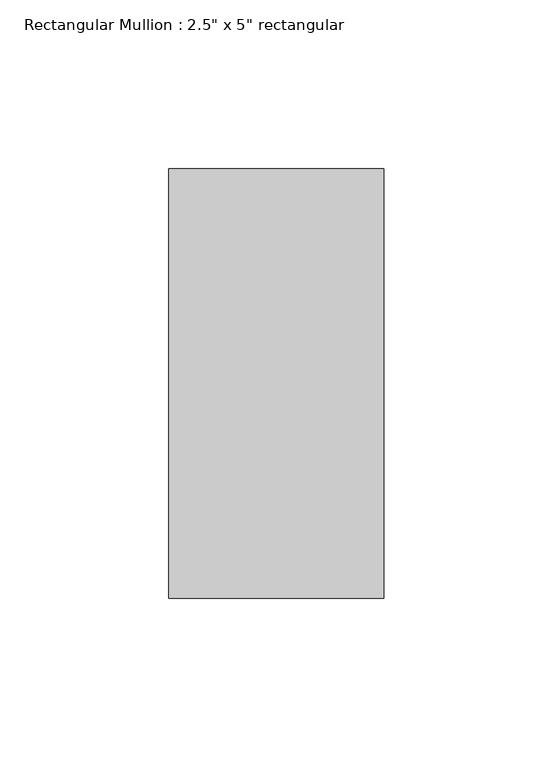
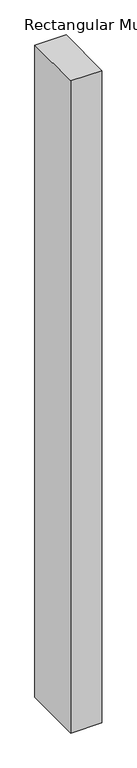
"""IFC4 building model written with IfcOpenShell, lengths in millimetres: member geometry."""

from ifc_helpers import new_model, si_unit, frame, origin, place, context, project, spatial, polyline, outline, extrude, source, transform, mapped, element, save


def member_647c50ce(model_context):
    return source(origin(), model_context, "Body", "SweptSolid", [
        extrude(outline(polyline([(0.0, 63.5), (0.0, -63.5), (-63.5, -63.5), (-63.5, 63.5), (0.0, 63.5)])), frame((0.0, 0.0, -1408.187673), z_axis=(0.0, 0.0, 1.0), x_axis=(1.0, 0.0, 0.0)), (0.0, 0.0, 1.0), 1408.187673),
    ])


if __name__ == "__main__":
    model = new_model("IFC4")
    model_context = context("Model", 3, world=origin())
    ifc_project = project(units=[si_unit("LENGTHUNIT", "METRE", prefix="MILLI")], contexts=[model_context])
    site = spatial("IfcSite", under=ifc_project)
    building = spatial("IfcBuilding", under=site)
    placement = place(None, origin())
    member_shape = member_647c50ce(model_context)
    element("IfcMember", 1, ObjectType="Rectangular Mullion : 2.5\" x 5\" rectangular", at=placement, inside=building, context=model_context, shape_type="MappedRepresentation", body=[
        mapped(member_shape, transform((0.0, 0.0, 0.0), x_axis=(1.0, 0.0, 0.0), y_axis=(0.0, 1.0, 0.0), z_axis=(0.0, 0.0, 1.0))),
    ])
    save(model, "model.ifc")

# Revit data of these elements
# Type "Rectangular Mullion : 2.5\" x 5\" rectangular"
#   built-in parameter 1007304 = 0.416667 (stored number, unit not read)
#   built-in parameter 1007301 = 0.104167 (stored number, unit not read)
#   built-in parameter 1007300 = 0.104167 (stored number, unit not read)
# Element 1 (IfcMember, "Rectangular Mullion : 2.5\" x 5\" rectangular")
#   Materials on its faces: "Aluminum"
# Materials
#   "Aluminum": class "Metal", colour RGB 247 247 247, transparency 0, Description = "Aluminum 6061", Cost = 0
